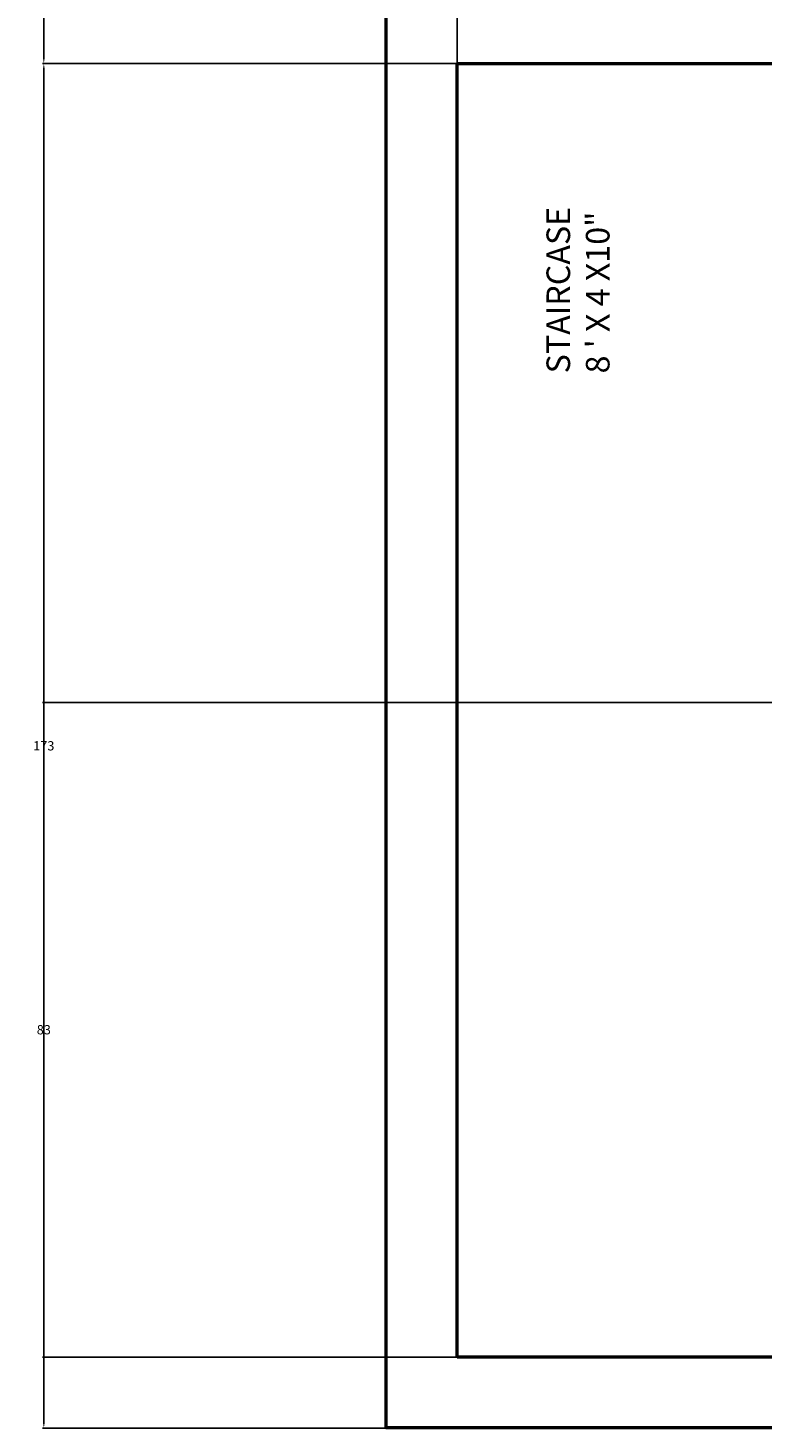
# Model space of a CAD drawing. Units: inches. Extents: x 3506 to 3958, y 1553 to 2506.
# Tile 1 of 16: x 3506 to 3599, y 1597 to 1775. Entities that reach past the tile are written whole.
import ezdxf

# ---------------------------------------------------------------- set-up
doc = ezdxf.new("R2010")
doc.units = ezdxf.units.IN
doc.header["$MEASUREMENT"] = 0
for name, color, linetype, lineweight in [('A-ANNO-DIMS', 2, 'Continuous', 18), ('A-AREA-IDEN', 7, 'Continuous', 18), ('A-WALL', 7, 'Continuous', 50)]:
    doc.layers.add(name, color=color, linetype=linetype, lineweight=lineweight)
doc.layers.add('A-WALL-PATT', color=251, linetype='Continuous', lineweight=13, true_color=0x636466)
doc.styles.get("Standard").update_dxf_attribs({"font": 'arial.ttf'})
doc.dimstyles.get("Standard").update_dxf_attribs({"dimtxt": 1.18, "dimasz": 0.68, "dimexe": 0.18, "dimexo": 0.0625, "dimgap": 0.09, "dimtad": 0, "dimtih": 1, "dimtoh": 1, "dimdec": 1, "dimzin": 0, "dimdsep": 46, "dimlunit": 3, "dimtxsty": 'Standard', "dimcen": 0.09, "dimadec": 0, "dimazin": 0, "dimtfac": 1, "dimtdec": 1, "dimtofl": 0, "dimtmove": 0, "dimatfit": 3, "dimfxl": 1, "dimtolj": 1, "dimtzin": 0, "dimarcsym": 0})

# ---------------------------------------------------------------- blocks, each defined once
blk = doc.blocks.new('*D41')
at = {"layer": 'A-ANNO-DIMS', "color": 0, "lineweight": -2, "transparency": 16777216}
for p, q in [((3560.67, 1770.39), (3508.1, 1770.39)), ((3508.28, 1769.71), (3508.28, 1684.59)), ((3508.28, 1598.07), (3508.28, 1683.2)), ((3551.67, 1597.39), (3508.1, 1597.39))]:
    blk.add_line(p, q, dxfattribs=at)
at = {"layer": 'A-ANNO-DIMS', "color": 0, "transparency": 16777216}
for points in [[(3508.17, 1769.71), (3508.39, 1769.71), (3508.28, 1770.39)], [(3508.17, 1598.07), (3508.39, 1598.07), (3508.28, 1597.39)]]:
    blk.add_solid(points, dxfattribs=at)
at = {"layer": 'Defpoints', "color": 0, "transparency": 16777216}
for p in [(3508.28, 1770.39), (3560.73, 1770.39), (3551.73, 1597.39)]:
    blk.add_point(p, dxfattribs=at)
at = {"layer": 'A-ANNO-DIMS', "color": 0, "transparency": 16777216, "insert": (3508.28, 1683.89), "char_height": 1.18, "attachment_point": 5}
blk.add_mtext('\\A1;173', dxfattribs=at)
blk = doc.blocks.new('*D42')
at = {"layer": 'A-ANNO-DIMS', "color": 0, "lineweight": -2, "transparency": 16777216}
for p, q in [((3560.67, 2000.39), (3508.1, 2000.39)), ((3508.28, 1999.71), (3508.28, 1886.09)), ((3508.28, 1771.07), (3508.28, 1884.7)), ((3560.67, 1770.39), (3508.1, 1770.39))]:
    blk.add_line(p, q, dxfattribs=at)
at = {"layer": 'A-ANNO-DIMS', "color": 0, "transparency": 16777216}
for points in [[(3508.17, 1999.71), (3508.39, 1999.71), (3508.28, 2000.39)], [(3508.17, 1771.07), (3508.39, 1771.07), (3508.28, 1770.39)]]:
    blk.add_solid(points, dxfattribs=at)
at = {"layer": 'Defpoints', "color": 0, "transparency": 16777216}
for p in [(3508.28, 2000.39), (3560.73, 2000.39), (3560.73, 1770.39)]:
    blk.add_point(p, dxfattribs=at)
at = {"layer": 'A-ANNO-DIMS', "color": 0, "transparency": 16777216, "insert": (3508.28, 1885.39), "char_height": 1.18, "attachment_point": 5}
blk.add_mtext('\\A1;230', dxfattribs=at)
blk = doc.blocks.new('*D51')
at = {"layer": 'A-ANNO-DIMS', "color": 0, "lineweight": -2, "transparency": 16777216}
for p, q in [((3608.67, 1689.39), (3508.1, 1689.39)), ((3508.28, 1688.71), (3508.28, 1648.59)), ((3508.28, 1607.07), (3508.28, 1647.2)), ((3608.67, 1606.39), (3508.1, 1606.39))]:
    blk.add_line(p, q, dxfattribs=at)
at = {"layer": 'A-ANNO-DIMS', "color": 0, "transparency": 16777216}
for points in [[(3508.17, 1688.71), (3508.39, 1688.71), (3508.28, 1689.39)], [(3508.17, 1607.07), (3508.39, 1607.07), (3508.28, 1606.39)]]:
    blk.add_solid(points, dxfattribs=at)
at = {"layer": 'Defpoints', "color": 0, "transparency": 16777216}
for p in [(3508.28, 1689.39), (3608.73, 1689.39), (3608.73, 1606.39)]:
    blk.add_point(p, dxfattribs=at)
at = {"layer": 'A-ANNO-DIMS', "color": 0, "transparency": 16777216, "insert": (3508.28, 1647.89), "char_height": 1.18, "attachment_point": 5}
blk.add_mtext('\\A1;83', dxfattribs=at)
blk = doc.blocks.new('*D52')
at = {"layer": 'A-ANNO-DIMS', "color": 0, "lineweight": -2, "transparency": 16777216}
for p, q in [((3560.73, 1606.46), (3560.73, 2505.02)), ((3561.41, 2504.84), (3583.77, 2504.84)), ((3608.05, 2504.84), (3585.69, 2504.84)), ((3608.73, 1606.46), (3608.73, 2505.02))]:
    blk.add_line(p, q, dxfattribs=at)
at = {"layer": 'A-ANNO-DIMS', "color": 0, "transparency": 16777216}
for points in [[(3561.41, 2504.96), (3561.41, 2504.73), (3560.73, 2504.84)], [(3608.05, 2504.96), (3608.05, 2504.73), (3608.73, 2504.84)]]:
    blk.add_solid(points, dxfattribs=at)
at = {"layer": 'Defpoints', "color": 0, "transparency": 16777216}
for p in [(3608.73, 2504.84), (3560.73, 1606.39), (3608.73, 1606.39)]:
    blk.add_point(p, dxfattribs=at)
at = {"layer": 'A-ANNO-DIMS', "color": 0, "transparency": 16777216, "insert": (3584.73, 2504.84), "char_height": 1.18, "attachment_point": 5}
blk.add_mtext('\\A1;48', dxfattribs=at)
blk = doc.blocks.new('*D63')
at = {"layer": 'A-ANNO-DIMS', "color": 0, "lineweight": -2, "transparency": 16777216}
for p, q in [((3869.67, 1800.46), (3508.1, 1800.46)), ((3508.28, 1799.78), (3508.28, 1786.12)), ((3508.28, 1771.07), (3508.28, 1784.74)), ((3869.67, 1770.39), (3508.1, 1770.39))]:
    blk.add_line(p, q, dxfattribs=at)
at = {"layer": 'A-ANNO-DIMS', "color": 0, "transparency": 16777216}
for points in [[(3508.17, 1799.78), (3508.39, 1799.78), (3508.28, 1800.46)], [(3508.17, 1771.07), (3508.39, 1771.07), (3508.28, 1770.39)]]:
    blk.add_solid(points, dxfattribs=at)
at = {"layer": 'Defpoints', "color": 0, "transparency": 16777216}
for p in [(3869.73, 1800.46), (3508.28, 1770.39), (3869.73, 1770.39)]:
    blk.add_point(p, dxfattribs=at)
at = {"layer": 'A-ANNO-DIMS', "color": 0, "transparency": 16777216, "insert": (3508.28, 1785.43), "char_height": 1.18, "attachment_point": 5}
blk.add_mtext('\\A1;30.07', dxfattribs=at)

msp = doc.modelspace()

# ---------------------------------------------------------------- hatches: boundary and pattern name
at = {"layer": 'A-WALL-PATT'}
h = msp.add_hatch(dxfattribs=at)
h.set_pattern_fill('ANSI31', color=256)
h.paths.add_polyline_path([(3911.7302, 2461.3942), (3551.7302, 2461.3942), (3551.7302, 2152.516), (3560.7302, 2152.516), (3560.7302, 2116.516), (3551.7302, 2116.516), (3551.7302, 1920.5711), (3556.2302, 1920.5711), (3560.7302, 1920.5711), (3560.7302, 2000.3942), (3692.7302, 2000.3942), (3692.7302, 1997.3942), (3697.7302, 1997.3942), (3697.7302, 2000.3942), (3771.7302, 2000.3942), (3771.7302, 1997.3942), (3776.7302, 1997.3942), (3776.7302, 1997.7206), (3778.5802, 1997.7206), (3807.5802, 1997.7206), (3807.5802, 1996.4519), (3778.5802, 1996.4519), (3778.5802, 1997.7206), (3776.7302, 1997.7206), (3776.7302, 1997.3942), (3771.7302, 1997.3942), (3771.7302, 2000.3942), (3697.7302, 2000.3942), (3697.7302, 1997.3942), (3692.7302, 1997.3942), (3689.8302, 1997.3942), (3689.8302, 1995.8192), (3653.8302, 1995.8192), (3653.8302, 1997.3942), (3689.8302, 1997.3942), (3692.7302, 1997.3942), (3692.7302, 2000.3942), (3560.7302, 2000.3942), (3560.7302, 1920.5711), (3551.7302, 1920.5711), (3551.7302, 1884.5711), (3551.7302, 1597.3942), (3911.7302, 1597.3942)], flags=17)
h.paths.add_polyline_path([(3596.7302, 2005.3942), (3596.7302, 2057.3035, -0.38730371), (3569.1778, 2085), (3569.15, 2085), (3569.15, 2086.2688), (3598.15, 2086.2688), (3598.15, 2085), (3569.1778, 2085, 0.38730371), (3596.7302, 2057.3035), (3596.7302, 2057.3942), (3601.7302, 2057.3942), (3601.7302, 2055.3942), (3630.7302, 2055.3942), (3630.7302, 2034.3942), (3694.7302, 2034.3942), (3694.7302, 2053.3942), (3699.7302, 2053.3942), (3699.7302, 2005.3942), (3860.7302, 2005.3942), (3860.7302, 2173.3942), (3771.7302, 2173.3942), (3771.7302, 2194.3942), (3776.7302, 2194.3942), (3776.7302, 2178.3942), (3860.7302, 2178.3942), (3860.7302, 2231.3942), (3601.7302, 2231.3942), (3601.7302, 2241.426), (3596.7302, 2241.426), (3596.7302, 2231.3942), (3560.7302, 2231.3942), (3560.7302, 2315.3942), (3596.7302, 2315.3942), (3596.7302, 2312.3942), (3601.7302, 2312.3942), (3601.7302, 2315.3942), (3697.7302, 2315.3942), (3697.7302, 2413.3942), (3692.7302, 2413.3942), (3692.7302, 2320.3942), (3560.7302, 2320.3942), (3560.7302, 2452.3942), (3692.7302, 2452.3942), (3692.7302, 2449.3942), (3697.7302, 2449.3942), (3697.7302, 2452.3942), (3771.7302, 2452.3942), (3771.7302, 2449.3942), (3776.7302, 2449.3942), (3776.7302, 2452.3942), (3860.7302, 2452.3942), (3860.7302, 2437.2075), (3865.2302, 2437.2075), (3865.2302, 2413.2075), (3860.7302, 2413.2075), (3860.7302, 2367.6976), (3865.2302, 2367.6976), (3869.7302, 2367.6976), (3869.7302, 2319.6976), (3860.7302, 2319.6976), (3860.7302, 2211.6248), (3869.7302, 2211.6248), (3869.7302, 2187.6248), (3860.7302, 2187.6248), (3860.7302, 2138.4346), (3865.2302, 2138.4346), (3869.7302, 2138.4346), (3869.7302, 2090.4346), (3860.7302, 2090.4346), (3860.7302, 1985.8449), (3869.7302, 1985.8449), (3869.7302, 1961.8449), (3860.7302, 1961.8449), (3860.7302, 1897.0756), (3865.2302, 1897.0756), (3869.7302, 1897.0756), (3869.7302, 1849.0756), (3860.7302, 1849.0756), (3860.7302, 1847.8112), (3860.7302, 1779.3942), (3596.7302, 1779.3942), (3596.7302, 1831.3942), (3601.7302, 1831.3942), (3601.7302, 1828.3942), (3630.7302, 1828.3942), (3630.7302, 1808.3942), (3691.7302, 1808.3942), (3691.7302, 1815.3942), (3696.7302, 1815.3942), (3696.7302, 1779.3942), (3860.7302, 1779.3942), (3860.7302, 1947.3942), (3771.7302, 1947.3942), (3771.7302, 1968.3942), (3776.7302, 1968.3942), (3776.7302, 1952.3942), (3860.7302, 1952.3942), (3860.7302, 2005.3942)], flags=0)
h.paths.add_polyline_path([(3596.7302, 2038.8546), (3601.7302, 2038.8546), (3601.7302, 2014.8546), (3596.7302, 2014.8546)], flags=0)
h.paths.add_polyline_path([(3564.1688, 2107), (3564.1688, 2167), (3644.1688, 2167), (3644.1688, 2107)], flags=0)
h.paths.add_polyline_path([(3607.0972, 2052.0208), (3620.8472, 2052.0208, -0.41421356), (3621.9931, 2050.875), (3621.9931, 2025.6667, -0.41421356), (3620.8472, 2024.5208), (3607.0972, 2024.5208, -0.41421356), (3605.9514, 2025.6667), (3605.9514, 2050.875, -0.41421356)], flags=0)
h.paths.add_polyline_path([(3578.5688, 2115), (3565.3688, 2115), (3565.3688, 2135.8), (3578.5688, 2135.8), (3578.5688, 2138.2), (3565.3688, 2138.2), (3565.3688, 2159), (3580.5688, 2159), (3580.5688, 2153.8), (3593.7688, 2167), (3593.7688, 2151.8), (3578.5688, 2151.8)], flags=0)
h.paths.add_polyline_path([(3610.9167, 2050.875), (3620.0833, 2050.875, -0.41421356), (3620.8472, 2050.1111), (3620.8472, 2039.6076, -0.41421356), (3620.0833, 2038.8438), (3610.9167, 2038.8438, -0.41421356), (3610.1528, 2039.6076), (3610.1528, 2050.1111, -0.41421356)], flags=0)
h.paths.add_polyline_path([(3610.9167, 2037.6979), (3620.0833, 2037.6979, -0.41421356), (3620.8472, 2036.934), (3620.8472, 2026.4306, -0.41421356), (3620.0833, 2025.6667), (3610.9167, 2025.6667, -0.41421356), (3610.1528, 2026.4306), (3610.1528, 2036.934, -0.41421356)], flags=0)
h.paths.add_polyline_path([(3616.2639, 2044.7639, -1), (3614.7361, 2044.7639, -1)], flags=0)
h.paths.add_polyline_path([(3615.8819, 2044.7639, -1), (3615.1181, 2044.7639, -1)], flags=0)
h.paths.add_polyline_path([(3616.2639, 2031.7778, -1), (3614.7361, 2031.7778, -1)], flags=0)
h.paths.add_polyline_path([(3615.8819, 2031.7778, -1), (3615.1181, 2031.7778, -1)], flags=0)
h.paths.add_polyline_path([(3609.7539, 2021.7868), (3626.9586, 2021.7868), (3626.9586, 2008.8833), (3609.7539, 2008.8833)], flags=0)
h.paths.add_polyline_path([(3610.4708, 2021.07), (3621.2237, 2021.07), (3621.2237, 2009.6002), (3610.4708, 2009.6002)], flags=0)
h.paths.add_polyline_path([(3611.5461, 2019.9947), (3620.1484, 2019.9947), (3620.1484, 2010.6755), (3611.5461, 2010.6755)], flags=0)
h.paths.add_polyline_path([(3621.9405, 2021.07), (3626.2417, 2021.07), (3626.2417, 2009.6002), (3621.9405, 2009.6002)], flags=0)
h.paths.add_polyline_path([(3622.6574, 2020.3531), (3625.5248, 2020.3531), (3625.5248, 2017.4857), (3622.6574, 2017.4857)], flags=0)
h.paths.add_polyline_path([(3622.6574, 2016.7688), (3625.5248, 2016.7688), (3625.5248, 2010.317), (3622.6574, 2010.317)], flags=0)
h.paths.add_polyline_path([(3624.808, 2016.0519), (3624.808, 2013.9013), (3624.0911, 2013.9013), (3624.0911, 2013.1845), (3623.3743, 2013.1845), (3623.3743, 2013.9013), (3623.3743, 2016.0519)], flags=0)
h.paths.add_polyline_path([(3623.0158, 2012.8261), (3625.1664, 2012.8261), (3625.1664, 2012.1092), (3623.0158, 2012.1092)], flags=0)
h.paths.add_polyline_path([(3623.0158, 2011.7508), (3625.1664, 2011.7508), (3625.1664, 2011.0339), (3623.0158, 2011.0339)], flags=0)
h.paths.add_polyline_path([(3650.0591, 2031.8202), (3674.0368, 2031.8202), (3674.0368, 2012.638), (3669.2413, 2012.638), (3669.2413, 2011.8388), (3672.4383, 2011.8388), (3672.4383, 2011.0395), (3651.6576, 2011.0395), (3651.6576, 2011.8388), (3654.8546, 2011.8388), (3654.8546, 2012.638), (3650.0591, 2012.638)], flags=0)
h.paths.add_polyline_path([(3658.0517, 2024.6269, -1), (3651.6576, 2024.6269, -1)], flags=0)
h.paths.add_polyline_path([(3657.2524, 2024.6269, -1), (3652.4569, 2024.6269, -1)], flags=0)
h.paths.add_polyline_path([(3656.4532, 2024.6269, -1), (3653.2561, 2024.6269, -1)], flags=0)
h.paths.add_polyline_path([(3655.6539, 2024.6269, -1), (3654.0554, 2024.6269, -1)], flags=0)
h.paths.add_polyline_path([(3657.2524, 2017.4336, -1), (3652.4569, 2017.4336, -1)], flags=0)
h.paths.add_polyline_path([(3656.4532, 2017.4336, -1), (3653.2561, 2017.4336, -1)], flags=0)
h.paths.add_polyline_path([(3655.6539, 2017.4336, -1), (3654.0554, 2017.4336, -1)], flags=0)
h.paths.add_polyline_path([(3659.6502, 2027.8239), (3664.4457, 2027.8239), (3664.4457, 2015.0358), (3659.6502, 2015.0358)], flags=0)
h.paths.add_polyline_path([(3663.6465, 2027.0247), (3663.6465, 2015.8351), (3660.4494, 2015.8351), (3660.4494, 2027.0247)], flags=0)
h.paths.add_polyline_path([(3562.6688, 1945.5), (3642.6688, 1945.5), (3642.6688, 1885.5), (3562.6688, 1885.5)], flags=0)
h.paths.add_polyline_path([(3671.6391, 2024.6269, -1), (3666.8435, 2024.6269, -1)], flags=0)
h.paths.add_polyline_path([(3670.8398, 2024.6269, -1), (3667.6428, 2024.6269, -1)], flags=0)
h.paths.add_polyline_path([(3672.4383, 2017.4336, -1), (3666.0443, 2017.4336, -1)], flags=0)
h.paths.add_polyline_path([(3670.0405, 2024.6269, -1), (3668.442, 2024.6269, -1)], flags=0)
h.paths.add_polyline_path([(3671.6391, 2017.4336, -1), (3666.8435, 2017.4336, -1)], flags=0)
h.paths.add_polyline_path([(3670.8398, 2017.4336, -1), (3667.6428, 2017.4336, -1)], flags=0)
h.paths.add_polyline_path([(3592.2688, 1945.5), (3592.2688, 1930.3), (3577.0688, 1930.3), (3577.0688, 1893.5), (3563.8688, 1893.5), (3563.8688, 1914.3), (3577.0688, 1914.3), (3577.0688, 1916.7), (3563.8688, 1916.7), (3563.8688, 1937.5), (3579.0688, 1937.5), (3579.0688, 1932.3)], flags=0)
h.paths.add_polyline_path([(3670.0405, 2017.4336, -1), (3668.442, 2017.4336, -1)], flags=0)
h.paths.add_polyline_path([(3596.7302, 2283.3942), (3601.7302, 2283.3942), (3601.7302, 2265.426), (3599.2302, 2265.426), (3599.2302, 2241.426), (3596.7302, 2241.426), (3596.7302, 2265.426)], flags=0)
h.paths.add_polyline_path([(3596.7302, 1810.7006), (3601.7302, 1810.7006), (3601.7302, 1786.7006), (3596.7302, 1786.7006)], flags=0)
h.paths.add_polyline_path([(3560.7302, 1770.3942), (3738.7302, 1770.3942), (3738.7302, 1746.3942), (3738.7302, 1722.3942), (3748.7302, 1722.3942), (3748.7302, 1674.3942), (3560.7302, 1674.3942)], flags=0)
h.paths.add_polyline_path([(3728.7302, 1746.3942), (3728.7302, 1756.0642), (3738.7302, 1746.3942), (3728.7302, 1738.1582), (3728.7302, 1698.3942), (3591.2519, 1698.3942), (3591.2519, 1746.3942)], flags=0)
h.paths.add_polyline_path([(3771.7302, 2399.3942), (3771.7302, 2420.3942), (3776.7302, 2420.3942), (3776.7302, 2404.3942), (3776.7302, 2399.3942)], flags=0)
h.paths.add_polyline_path([(3911.7302, 2461.3942), (3551.7302, 2461.3942), (3551.7302, 2152.516), (3560.7302, 2152.516), (3560.7302, 2116.516), (3551.7302, 2116.516), (3551.7302, 1920.5711), (3560.7302, 1920.5711), (3560.7302, 2000.3942), (3692.7302, 2000.3942), (3692.7302, 1997.3942), (3697.7302, 1997.3942), (3697.7302, 2000.3942), (3771.7302, 2000.3942), (3771.7302, 1997.3942), (3776.7302, 1997.3942), (3776.7302, 1997.7206), (3778.5802, 1997.7206), (3807.5802, 1997.7206), (3807.5802, 1996.4519), (3778.5802, 1996.4519), (3778.5802, 1997.7206), (3776.7302, 1997.7206), (3776.7302, 1997.3942), (3771.7302, 1997.3942), (3771.7302, 2000.3942), (3697.7302, 2000.3942), (3697.7302, 1997.3942), (3692.7302, 1997.3942), (3689.8302, 1997.3942), (3689.8302, 1995.8192), (3653.8302, 1995.8192), (3653.8302, 1997.3942), (3689.8302, 1997.3942), (3692.7302, 1997.3942), (3692.7302, 2000.3942), (3560.7302, 2000.3942), (3560.7302, 1920.5711), (3551.7302, 1920.5711), (3551.7302, 1597.3942), (3911.7302, 1597.3942)], flags=17)

# ---------------------------------------------------------------- linework, layer by layer
at = {"layer": 'A-WALL'}
for p, q in [((3560.7302, 1606.3942), (3560.7302, 1770.3942)), ((3560.7302, 1770.3942), (3771.7302, 1770.3942)), ((3902.7302, 1606.3942), (3560.7302, 1606.3942))]:
    msp.add_line(p, q, dxfattribs=at)
msp.add_lwpolyline([(3551.7302, 2461.3942), (3911.7302, 2461.3942), (3911.7302, 1597.3942), (3551.7302, 1597.3942)], close=True, dxfattribs=at)

# ---------------------------------------------------------------- texts
at = {"layer": 'A-AREA-IDEN', "insert": (3572.0569, 1731.1037), "char_height": 3, "attachment_point": 1, "rotation": 90}
msp.add_mtext_dynamic_manual_height_columns('STAIRCASE\\P8 \' X 4 X10"', width=46.119714, gutter_width=1, heights=[0], dxfattribs=at)

# ---------------------------------------------------------------- dimensions: what is measured, and where the dimension line sits
at = {"layer": 'A-ANNO-DIMS'}
dim = msp.add_linear_dim(base=(3608.7302, 2504.8442), p1=(3560.7302, 1606.3942), p2=(3608.7302, 1606.3942), dimstyle='Standard', override={"dimdec": 0, "dimlfac": 1, "dimrnd": 0, "dimzin": 0, "dimdsep": 46, "dimlunit": 2}, dxfattribs=at)
dim.commit()
dim.dimension.update_dxf_attribs({"geometry": '*D52', "text_midpoint": (3584.7302, 2504.8442)})
for base, p1, p2, override, picture, middle in [((3508.2802, 2000.3942), (3560.7302, 1770.3942), (3560.7302, 2000.3942), {"dimdec": 0, "dimlfac": 1, "dimrnd": 0, "dimzin": 0, "dimdsep": 46, "dimlunit": 2}, '*D42', (3508.2802, 1885.3942)), ((3508.2802, 1770.3942), (3869.7302, 1800.4628), (3869.7302, 1770.3942), {"dimdec": 2, "dimlfac": 1, "dimrnd": 0, "dimzin": 0, "dimdsep": 46, "dimlunit": 2}, '*D63', (3508.2802, 1785.4285)), ((3508.2802, 1770.3942), (3551.7302, 1597.3942), (3560.7302, 1770.3942), {"dimdec": 0, "dimlfac": 1, "dimrnd": 0, "dimzin": 0, "dimdsep": 46, "dimlunit": 2}, '*D41', (3508.2802, 1683.8942)), ((3508.2802, 1689.3942), (3608.7302, 1606.3942), (3608.7302, 1689.3942), {"dimdec": 0, "dimlfac": 1, "dimrnd": 0, "dimzin": 0, "dimdsep": 46, "dimlunit": 2}, '*D51', (3508.2802, 1647.8942))]:
    dim = msp.add_linear_dim(base=base, p1=p1, p2=p2, angle=90, dimstyle='Standard', override=override, dxfattribs=at)
    dim.commit()
    dim.dimension.update_dxf_attribs({"geometry": picture, "text_midpoint": middle})

doc.saveas('drawing.dxf')
